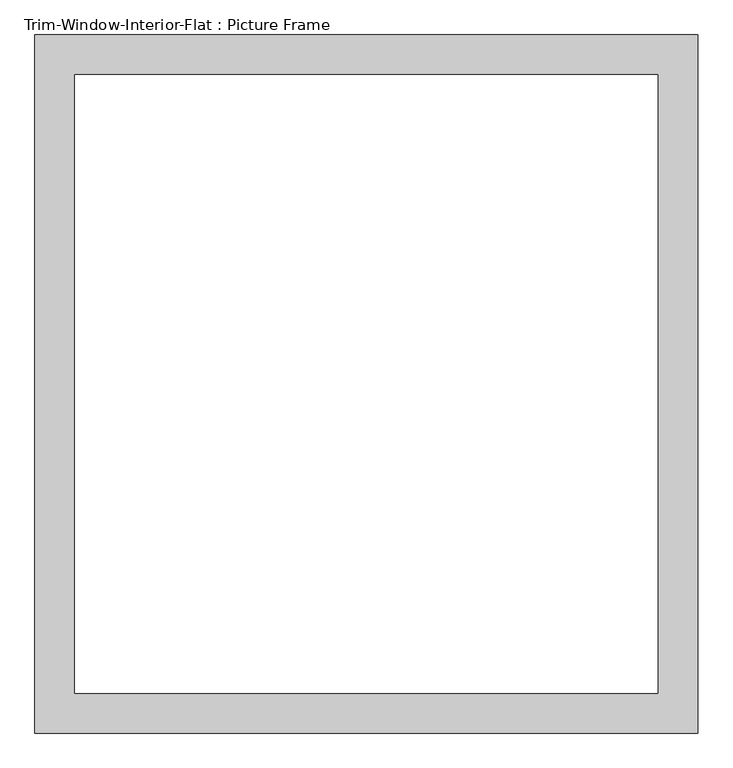
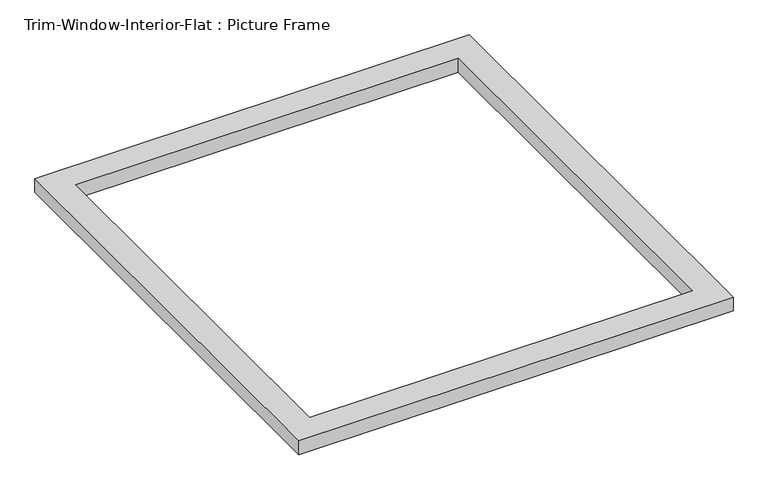
"""IFC4 building model written with IfcOpenShell, lengths in millimetres: proxy geometry, Trim-Window-Interior-Flat : Picture Frame."""

from ifc_helpers import new_model, si_unit, origin, origin_with_axes, place, context, project, spatial, polyline, outline, extrude, source, transform, mapped, element, save


def trim_window_interior_flat_picture_frame_1c9020d0(model_context):
    return source(origin(), model_context, "Body", "SweptSolid", [
        extrude(outline(polyline([(476.25, -44.45), (-476.25, -44.45), (-476.25, 958.85), (476.25, 958.85), (476.25, -44.45)]), holes=[polyline([(419.1, 12.7), (419.1, 901.7), (-419.1, 901.7), (-419.1, 12.7), (419.1, 12.7)])]), origin_with_axes(), (0.0, 0.0, 1.0), 31.75),
    ])


if __name__ == "__main__":
    model = new_model("IFC4")
    model_context = context("Model", 3, world=origin())
    ifc_project = project(units=[si_unit("LENGTHUNIT", "METRE", prefix="MILLI")], contexts=[model_context])
    site = spatial("IfcSite", under=ifc_project)
    building = spatial("IfcBuilding", under=site)
    placement = place(None, origin())
    trim_window_interior_flat_picture_frame_shape = trim_window_interior_flat_picture_frame_1c9020d0(model_context)
    element("IfcBuildingElementProxy", 1, Name="Trim-Window-Interior-Flat : Picture Frame", ObjectType="Trim-Window-Interior-Flat : Picture Frame", at=placement, inside=building, context=model_context, shape_type="MappedRepresentation", body=[
        mapped(trim_window_interior_flat_picture_frame_shape, transform((0.0, 0.0, 0.0), x_axis=(1.0, 0.0, 0.0), y_axis=(0.0, 1.0, 0.0), z_axis=(0.0, 0.0, 1.0))),
    ])
    save(model, "model.ifc")

# Revit data of these elements
# Type "Trim-Window-Interior-Flat : Picture Frame"
#   Trim Thickness_Picture Frame = 0' - 1 1/4"
#   Trim Width = 0' - 2 1/4"
#   Trim Thickness_with Sill = 0' - 0 3/4"
#   Sill Thickness = 0' - 1 1/4"
#   Opening Width [instance default] = 2' - 0"
#   Opening Height [instance default] = 3' - 0"
#   Default Elevation = 4' - 0"
#   Sill = no
#   Picture Frame = yes
#   Trim Material [instance default] = none
# Element 1 (IfcBuildingElementProxy, "Trim-Window-Interior-Flat : Picture Frame")
#   Opening Width = 2' - 10"
#   Trim Material = Wood - Stained
#   Materials on its faces: "Wood - Stained"
# Materials
#   "Wood - Stained": class "Wood", colour RGB 224 178 126, transparency 0, Cost = 0
